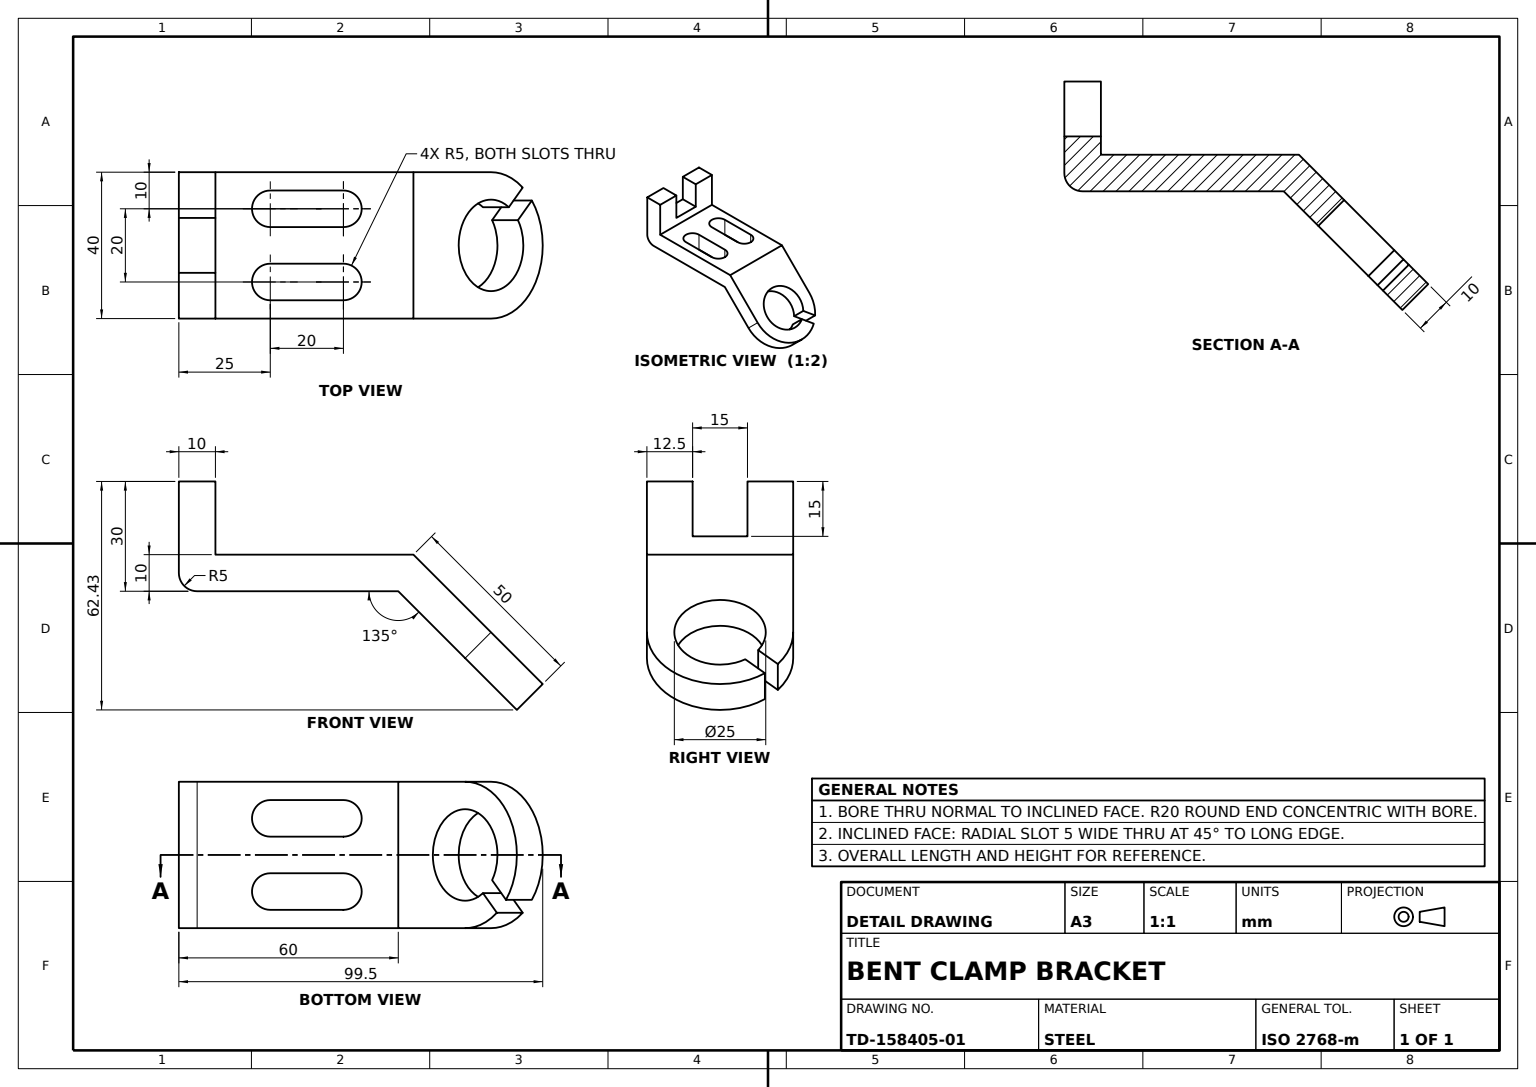
from build123d import *

# Parameters (mm, degrees)
ANGLED_BRACKET_BODY_DEPTH   = 20
GUIDE_UPRIGHT_BOSS_DEPTH    = 10
GUIDE_NOTCH_15X15_REACH     = 99.269
GUIDE_NOTCH_SKETCH_W        = 15
GUIDE_NOTCH_SKETCH_H        = 15
GUIDE_SLOTS_REACH           = 111.999
ANGLED_TRIM_CUT_45DEG_DEPTH = 96.535099634


with BuildPart() as part:
    # Bracket Profile Sketch → Angled Bracket Body (new, symmetric)
    with BuildSketch(Plane.XY):
        with BuildLine():
            Line((0, 5), (0, 30))
            Line((0, 30), (-10, 30))
            Line((-10, 30), (-10, 10))
            Line((-10, 10), (-64.142135624, 10))
            Line((-64.142135624, 10), (-85.355339059, -11.213203436))
            Line((-85.355339059, -11.213203436), (-78.284271247, -18.284271247))
            Line((-78.284271247, -18.284271247), (-60, 0))
            Line((-60, 0), (-5, 0))
            ThreePointArc((-5, 0), (-1.464466094, 1.464466094), (0, 5))
        make_face()
    extrude(amount=ANGLED_BRACKET_BODY_DEPTH, both=True)

    # Guide Upright Sketch → Guide Upright Boss (add)
    with BuildSketch(Plane(origin=(-37.071067812, 37.071067812, 0), x_dir=(0, 0, 1), z_dir=(-0.7071067811865486, 0.7071067811865465, 0))):
        with BuildLine():
            Line((-20, -68.284271247), (20, -68.284271247))
            ThreePointArc((20, -68.284271247), (0, -88.284271247), (-20, -68.284271247))
        make_face()
    extrude(amount=-GUIDE_UPRIGHT_BOSS_DEPTH)

    # Guide Notch Sketch → Guide Notch 15x15 (cut, up to next)
    with BuildSketch(Plane.ZY.offset(10), mode=Mode.PRIVATE) as guide_notch_15x15_sk1:
        with Locations((0, 22.5)):
            Rectangle(GUIDE_NOTCH_SKETCH_W, GUIDE_NOTCH_SKETCH_H)
    guide_notch_15x15_tool1 = extrude(guide_notch_15x15_sk1.sketch, amount=-GUIDE_NOTCH_15X15_REACH, mode=Mode.PRIVATE) & part.part
    add(guide_notch_15x15_tool1.solids().sort_by_distance((-10, 22.5, 0))[0], mode=Mode.SUBTRACT)

    # Guide Slots Sketch → Guide Slots (cut, up to next)
    with BuildSketch(Plane(origin=(0, 10, 0), x_dir=(1, 0, 0), z_dir=(0, 1, 0)), mode=Mode.PRIVATE) as guide_slots_sk1:
        with BuildLine():
            Line((-45, 15), (-25, 15))
            ThreePointArc((-25, 15), (-20, 10), (-25, 5))
            Line((-25, 5), (-45, 5))
            ThreePointArc((-45, 5), (-50, 10), (-45, 15))
        make_face()
    guide_slots_tool1 = extrude(guide_slots_sk1.sketch, amount=-GUIDE_SLOTS_REACH, mode=Mode.PRIVATE) & part.part
    # Guide Slots Sketch → Guide Slots (cut, up to next)
    with BuildSketch(Plane(origin=(0, 10, 0), x_dir=(1, 0, 0), z_dir=(0, 1, 0)), mode=Mode.PRIVATE) as guide_slots_sk2:
        with BuildLine():
            Line((-45, -15), (-25, -15))
            ThreePointArc((-25, -15), (-20, -10), (-25, -5))
            Line((-25, -5), (-45, -5))
            ThreePointArc((-45, -5), (-50, -10), (-45, -15))
        make_face()
    guide_slots_tool2 = extrude(guide_slots_sk2.sketch, amount=-GUIDE_SLOTS_REACH, mode=Mode.PRIVATE) & part.part
    add(guide_slots_tool1.solids().sort_by_distance((-35, 10, -10))[0], mode=Mode.SUBTRACT)
    add(guide_slots_tool2.solids().sort_by_distance((-35, 10, 10))[0], mode=Mode.SUBTRACT)

    # Angled Trim Sketch → Angled Trim Cut 45deg (cut, through all)
    with BuildSketch(Plane(origin=(-37.071067812, 37.071067812, 0), x_dir=(0, 0, 1), z_dir=(-0.7071067811865486, 0.7071067811865465, 0))):
        with BuildLine():
            Line((6.892487085, -78.712292238), (12.91897827, -84.738783423))
            Line((12.91897827, -84.738783423), (16.464043435, -81.212780777))
            Line((16.464043435, -81.212780777), (10.428020991, -75.176758332))
            ThreePointArc((10.428020991, -75.176758332), (-8.838834765, -59.445436483), (6.892487085, -78.712292238))
        make_face()
    extrude(amount=-ANGLED_TRIM_CUT_45DEG_DEPTH, mode=Mode.SUBTRACT)


solid = part.part
